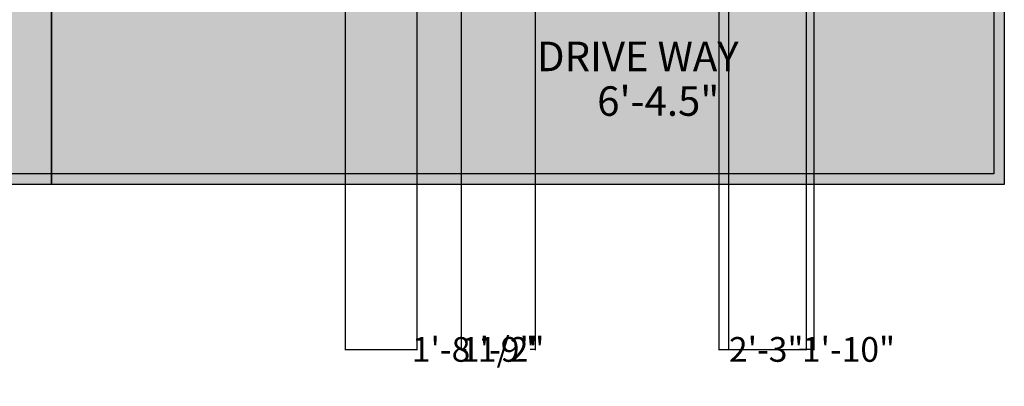
# Model space of a CAD drawing. Units: inches. Extents: x 1884 to 2398, y 474 to 1488.
# Tile 2 of 39: x 2118 to 2397, y 474 to 577. Entities that reach past the tile are written whole.
import ezdxf

# ---------------------------------------------------------------- set-up
doc = ezdxf.new("R2010")
doc.units = ezdxf.units.IN
doc.header["$MEASUREMENT"] = 0
for name, color, linetype, lineweight in [('A-ANNO-DIMS', 2, 'Continuous', 18), ('A-AREA-IDEN', 7, 'Continuous', 18), ('A-WALL-PATT', 250, 'Continuous', 13), ('C-PROP', 7, 'Continuous', 30), ('L-TURF-PATT', 73, 'Continuous', 13), ('walls', 7, 'Continuous', 35)]:
    doc.layers.add(name, color=color, linetype=linetype, lineweight=lineweight)
doc.layers.add('L-PVMT-PATT', color=9, linetype='Continuous', lineweight=13, true_color=0xc7c8ca)
doc.styles.get("Standard").update_dxf_attribs({"font": 'arial.ttf'})
doc.dimstyles.get("Standard").update_dxf_attribs({"dimtxt": 7, "dimasz": 0.18, "dimexe": 0.18, "dimexo": 0.0625, "dimgap": 0.09, "dimtad": 0, "dimtih": 1, "dimtoh": 1, "dimzin": 0, "dimdsep": 46, "dimlunit": 3, "dimtxsty": 'Standard', "dimcen": 0.09, "dimadec": 0, "dimazin": 0, "dimtfac": 1, "dimtofl": 0, "dimtmove": 0, "dimatfit": 3, "dimfxl": 1, "dimtolj": 1, "dimtzin": 0, "dimarcsym": 0})

# ---------------------------------------------------------------- blocks, each defined once
blk = doc.blocks.new('*D44')
at = {"layer": 'A-ANNO-DIMS', "color": 0, "lineweight": -2, "transparency": 16777216}
for p, q in [((2209.76, 1247.82), (2209.76, 484)), ((2230.03, 1247.82), (2230.03, 484)), ((2209.94, 484.18), (2229.85, 484.18)), ((2230.03, 484.18), (2230.21, 484.18))]:
    blk.add_line(p, q, dxfattribs=at)
at = {"layer": 'A-ANNO-DIMS', "color": 0, "lineweight": 100, "transparency": 16777216}
for points in [[(2209.94, 484.21), (2209.94, 484.15), (2209.76, 484.18)], [(2229.85, 484.21), (2229.85, 484.15), (2230.03, 484.18)]]:
    blk.add_solid(points, dxfattribs=at)
at = {"layer": 'Defpoints', "color": 0, "lineweight": 100, "transparency": 16777216}
for p in [(2209.76, 1247.88), (2230.03, 1247.88), (2230.03, 484.18)]:
    blk.add_point(p, dxfattribs=at)
at = {"layer": 'A-ANNO-DIMS', "color": 0, "transparency": 16777216, "insert": (2247.43, 484.18), "char_height": 7, "attachment_point": 5}
blk.add_mtext('\\A1;1\'-8 1/2"', dxfattribs=at)
blk = doc.blocks.new('*D45')
at = {"layer": 'A-ANNO-DIMS', "color": 0, "lineweight": -2, "transparency": 16777216}
for p, q in [((2242.62, 1322.82), (2242.62, 484)), ((2263.62, 1322.82), (2263.62, 484)), ((2242.8, 484.18), (2244.05, 484.18)), ((2263.44, 484.18), (2262.18, 484.18))]:
    blk.add_line(p, q, dxfattribs=at)
at = {"layer": 'A-ANNO-DIMS', "color": 0, "lineweight": 100, "transparency": 16777216}
for points in [[(2242.8, 484.21), (2242.8, 484.15), (2242.62, 484.18)], [(2263.44, 484.21), (2263.44, 484.15), (2263.62, 484.18)]]:
    blk.add_solid(points, dxfattribs=at)
at = {"layer": 'Defpoints', "color": 0, "lineweight": 100, "transparency": 16777216}
for p in [(2242.62, 1322.88), (2263.62, 1322.88), (2263.62, 484.18)]:
    blk.add_point(p, dxfattribs=at)
at = {"layer": 'A-ANNO-DIMS', "color": 0, "transparency": 16777216, "insert": (2253.12, 484.18), "char_height": 7, "attachment_point": 5}
blk.add_mtext('\\A1;1\'-9"', dxfattribs=at)
blk = doc.blocks.new('*D47')
at = {"layer": 'A-ANNO-DIMS', "color": 0, "lineweight": -2, "transparency": 16777216}
for p, q in [((2315.59, 959.7), (2315.59, 484)), ((2342.53, 959.7), (2342.53, 484)), ((2315.77, 484.18), (2319.61, 484.18)), ((2342.35, 484.18), (2338.51, 484.18))]:
    blk.add_line(p, q, dxfattribs=at)
at = {"layer": 'A-ANNO-DIMS', "color": 0, "lineweight": 100, "transparency": 16777216}
for points in [[(2315.77, 484.21), (2315.77, 484.15), (2315.59, 484.18)], [(2342.35, 484.21), (2342.35, 484.15), (2342.53, 484.18)]]:
    blk.add_solid(points, dxfattribs=at)
at = {"layer": 'Defpoints', "color": 0, "lineweight": 100, "transparency": 16777216}
for p in [(2315.59, 959.77), (2342.53, 959.77), (2342.53, 484.18)]:
    blk.add_point(p, dxfattribs=at)
at = {"layer": 'A-ANNO-DIMS', "color": 0, "transparency": 16777216, "insert": (2329.06, 484.18), "char_height": 7, "attachment_point": 5}
blk.add_mtext('\\A1;2\'-3"', dxfattribs=at)
blk = doc.blocks.new('*D49')
at = {"layer": 'A-ANNO-DIMS', "color": 0, "lineweight": -2, "transparency": 16777216}
for p, q in [((2318.41, 987.72), (2318.41, 484)), ((2340.41, 987.72), (2340.41, 484)), ((2318.59, 484.18), (2340.23, 484.18)), ((2340.41, 484.18), (2340.59, 484.18))]:
    blk.add_line(p, q, dxfattribs=at)
at = {"layer": 'A-ANNO-DIMS', "color": 0, "lineweight": 100, "transparency": 16777216}
for points in [[(2318.59, 484.21), (2318.59, 484.15), (2318.41, 484.18)], [(2340.23, 484.21), (2340.23, 484.15), (2340.41, 484.18)]]:
    blk.add_solid(points, dxfattribs=at)
at = {"layer": 'Defpoints', "color": 0, "lineweight": 100, "transparency": 16777216}
for p in [(2318.41, 987.78), (2340.41, 987.78), (2340.41, 484.18)]:
    blk.add_point(p, dxfattribs=at)
at = {"layer": 'A-ANNO-DIMS', "color": 0, "transparency": 16777216, "insert": (2352.37, 484.18), "char_height": 7, "attachment_point": 5}
blk.add_mtext('\\A1;1\'-10"', dxfattribs=at)

msp = doc.modelspace()

# ---------------------------------------------------------------- hatches: boundary and pattern name
at = {"layer": 'A-WALL-PATT'}
h = msp.add_hatch(color=256, dxfattribs=at)
h.dxf.hatch_style = 1
h.paths.add_polyline_path([(2351.529, 837.963), (2342.529, 837.963), (2342.529, 813.478), (2351.529, 813.478)])
h.paths.add_polyline_path([(2351.529, 782.175), (2342.529, 782.175), (2342.529, 778.966), (2238.447, 778.966), (2238.447, 769.966), (2351.529, 769.966)])
h.paths.add_polyline_path([(2351.529, 914.773), (2342.529, 914.773), (2342.529, 901.966), (2222.529, 901.966), (2222.529, 908.236), (2213.529, 908.236), (2213.529, 901.966), (2198.529, 901.966), (2198.529, 892.966), (2198.529, 815.857), (2203.029, 815.857), (2203.029, 892.966), (2342.529, 892.966), (2342.529, 869.555), (2346.047, 869.555), (2351.529, 869.555), (2351.529, 880.385)])
h.paths.add_polyline_path([(2208.948, 778.966), (2203.029, 778.966), (2203.029, 782.647), (2198.529, 782.647), (2198.529, 779.109), (2193.526, 779.109), (2193.526, 769.966), (2198.529, 769.966), (2208.948, 769.966)])
h.paths.add_polyline_path([(2126.529, 815.801), (2117.529, 815.801), (2117.529, 676.183), (2126.529, 676.183), (2126.529, 769.966), (2132.515, 769.966), (2132.515, 778.664), (2126.529, 778.664)])
h.paths.add_polyline_path([(2135.996, 901.385), (2009.529, 901.385), (2009.529, 929.544), (2000.529, 929.544), (2000.529, 892.385), (2117.529, 892.385), (2117.529, 880.382), (2126.529, 880.382), (2126.529, 892.385), (2135.996, 892.385)])
h.paths.add_polyline_path([(2198.529, 901.385), (2185.2, 901.385), (2185.2, 892.385), (2198.529, 892.385), (2198.529, 892.966)])
h.paths.add_polyline_path([(1961.529, 892.385), (1965.143, 892.385), (1965.143, 901.385), (1952.529, 901.385), (1952.529, 604.13), (1961.529, 604.13), (1961.529, 631.385), (1988.002, 631.385), (1988.002, 640.385), (1961.529, 640.385)])
h.paths.add_polyline_path([(1955.529, 604.13), (1952.529, 604.13), (1952.529, 530.885), (2126.529, 530.885), (2126.529, 533.885), (1955.529, 533.885)])
h.paths.add_polyline_path([(2396.529, 604.13), (2393.529, 604.13), (2393.529, 533.885), (2126.529, 533.885), (2126.529, 530.885), (2396.529, 530.885)])
h.paths.add_polyline_path([(2396.529, 779.322), (2387.529, 779.322), (2387.529, 604.13), (2396.529, 604.13)])
at = {"layer": 'L-PVMT-PATT'}
h = msp.add_hatch(color=256, dxfattribs=at)
h.dxf.hatch_style = 1
h.paths.add_polyline_path([(2387.529, 769.966), (2351.529, 769.966), (2238.447, 769.966), (2238.447, 762.15), (2238.447, 754.445), (2126.529, 754.445), (2126.529, 676.183), (2134.868, 676.183), (2142.673, 676.183), (2142.673, 646.578), (2134.868, 646.578), (2126.529, 646.578), (2126.529, 640.17), (2387.529, 640.17)])
h.paths.add_polyline_path([(2387.529, 631.385), (2303.086, 631.385), (2303.086, 615.671), (2387.529, 615.671)])
h.paths.add_polyline_path([(2387.529, 640.17), (2126.529, 640.17), (2126.529, 631.385), (2387.529, 631.385)])
h.paths.add_polyline_path([(2393.529, 604.13), (2387.529, 604.13), (2387.529, 615.671), (2303.086, 615.671), (2303.086, 607.943), (2249.649, 607.943), (2126.529, 607.943), (2126.529, 533.885), (2393.529, 533.885)])
h.paths.add_polyline_path([(2257.825, 611.008), (2257.83, 611.337), (2257.915, 616.493), (2258.021, 621.805), (2258.146, 627.274), (2258.252, 631.385), (2126.529, 631.385), (2126.529, 611.008)])
h.paths.add_polyline_path([(2258.892, 611.285), (2258.888, 611.008), (2300.247, 611.008), (2300.247, 631.385), (2259.314, 631.385), (2259.206, 627.173), (2259.081, 621.72), (2258.976, 616.424)])
at = {"layer": 'L-TURF-PATT'}
h = msp.add_hatch(color=256, dxfattribs=at)
h.dxf.hatch_style = 1
h.paths.add_polyline_path([(2126.529, 607.943), (2117.364, 607.943), (2117.364, 631.385), (1961.529, 631.385), (1961.529, 604.13), (1955.529, 604.13), (1955.529, 533.885), (2126.529, 533.885)])

# ---------------------------------------------------------------- linework, layer by layer
at = {"layer": 'C-PROP'}
for p, q in [((2396.529, 1406.885), (2396.529, 530.885)), ((2393.529, 604.13), (2393.529, 533.885)), ((2393.529, 533.885), (1955.529, 533.885)), ((2396.529, 530.885), (1952.529, 530.885))]:
    msp.add_line(p, q, dxfattribs=at)
at = {"layer": 'walls'}
msp.add_line((2126.529, 530.885), (2126.529, 769.966), dxfattribs=at)

# ---------------------------------------------------------------- texts
at = {"layer": 'A-AREA-IDEN'}
for s, p in [('DRIVE WAY', (2264.107, 562.921)), ('6\'-4.5"', (2281.168, 550.288))]:
    msp.add_text(s, height=8.3413, dxfattribs=at).set_placement(p)

# ---------------------------------------------------------------- dimensions: what is measured, and where the dimension line sits
at = {"layer": 'A-ANNO-DIMS'}
for base, p1, p2, picture, middle in [((2263.617, 484.185), (2242.617, 1322.885), (2263.617, 1322.885), '*D45', (2253.117, 484.185)), ((2230.029, 484.185), (2209.755, 1247.885), (2230.029, 1247.885), '*D44', (2247.429, 484.185)), ((2340.409, 484.185), (2318.409, 987.778), (2340.409, 987.778), '*D49', (2352.373, 484.185)), ((2342.529, 484.185), (2315.591, 959.766), (2342.529, 959.766), '*D47', (2329.06, 484.185))]:
    dim = msp.add_linear_dim(base=base, p1=p1, p2=p2, dimstyle='Standard', override={"dimdec": 1, "dimlfac": 1, "dimrnd": 0, "dimzin": 1, "dimdsep": 46, "dimlunit": 4, "dimfrac": 2}, dxfattribs=at)
    dim.commit()
    dim.dimension.update_dxf_attribs({"geometry": picture, "text_midpoint": middle})

doc.saveas('drawing.dxf')
